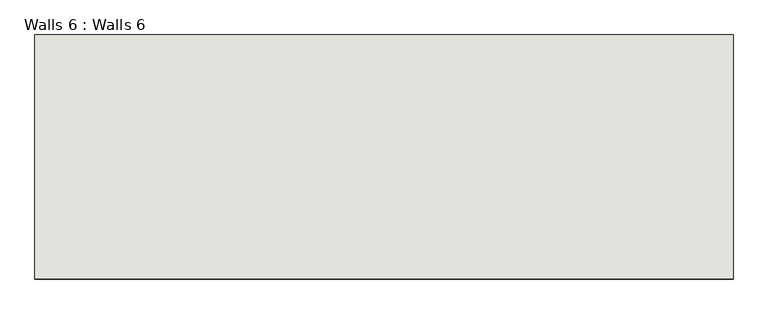
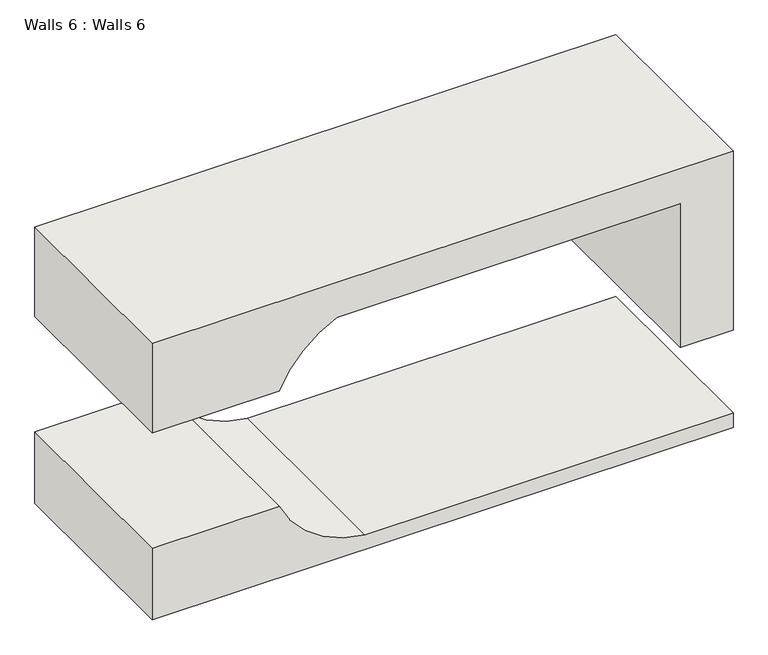
"""IFC4 building model written with IfcOpenShell, lengths in millimetres: wall geometry, Walls 6 : Walls 6."""

from ifc_helpers import new_model, si_unit, point, frame, frame_2d, origin, place, context, project, spatial, polyline, circle_curve, trimmed, segment, composite_curve, outline, extrude, source, transform, mapped, element, save


def walls_6_walls_6_38c579e2(model_context):
    return source(origin(), model_context, "Body", "SweptSolid", [
        extrude(outline(composite_curve([segment(polyline([(6096.0, -5912.2996792), (6096.0, -12313.0996792), (5054.6, -12313.0996792), (5054.6, -10914.4996792)]), True, "CONTINUOUS"), segment(trimmed(circle_curve(frame_2d((4512.0675118, -9736.967191)), 1296.5046322), [point((5054.6, -10914.4996792))], [point((5689.6, -10279.4996792))], True, "CARTESIAN"), True, "CONTINUOUS"), segment(polyline([(5689.6, -10279.4996792), (5689.6, -6494.8495402), (4013.2, -6494.8495402), (4013.2, -5912.2996792), (6096.0, -5912.2996792)]), True, "CONTINUOUS")], self_intersect=False)), frame((0.0, -7790.8651578, 0.0), z_axis=(0.0, 1.0, 0.0), x_axis=(0.0, 0.0, 1.0)), (0.0, 0.0, 1.0), 2237.7737639),
        extrude(outline(composite_curve([segment(polyline([(2876.6, -5912.2996792), (3048.0, -5912.2996792), (3048.0, -9971.3507355)]), True, "CONTINUOUS"), segment(trimmed(circle_curve(frame_2d((4203.6522485, -9864.9373205)), 1160.5412248), [point((3048.0, -9971.3507355))], [point((3708.4, -10914.4996792))], True, "CARTESIAN"), True, "CONTINUOUS"), segment(polyline([(3708.4, -10914.4996792), (3708.4, -12313.0996792), (2876.6, -12313.0996792), (2876.6, -5912.2996792)]), True, "CONTINUOUS")], self_intersect=False)), frame((0.0, -7790.8651578, 0.0), z_axis=(0.0, 1.0, 0.0), x_axis=(0.0, 0.0, 1.0)), (0.0, 0.0, 1.0), 2237.7737639),
    ])


if __name__ == "__main__":
    model = new_model("IFC4")
    model_context = context("Model", 3, world=origin())
    ifc_project = project(units=[si_unit("LENGTHUNIT", "METRE", prefix="MILLI")], contexts=[model_context])
    site = spatial("IfcSite", under=ifc_project)
    building = spatial("IfcBuilding", under=site)
    placement = place(None, origin())
    walls_6_walls_6_shape = walls_6_walls_6_38c579e2(model_context)
    element("IfcWall", 1, ObjectType="Walls 6 : Walls 6", at=placement, inside=building, context=model_context, shape_type="MappedRepresentation", body=[
        mapped(walls_6_walls_6_shape, transform((0.0, 0.0, 0.0), x_axis=(1.0, 0.0, 0.0), y_axis=(0.0, 1.0, 0.0), z_axis=(0.0, 0.0, 1.0))),
    ])
    save(model, "model.ifc")

# Revit data of these elements
# Element 1 (IfcWall, "Walls 6 : Walls 6")
#   Materials on its faces: "Default Wall"
# Materials
#   "Default Wall": colour RGB 80 80 80, transparency 0
